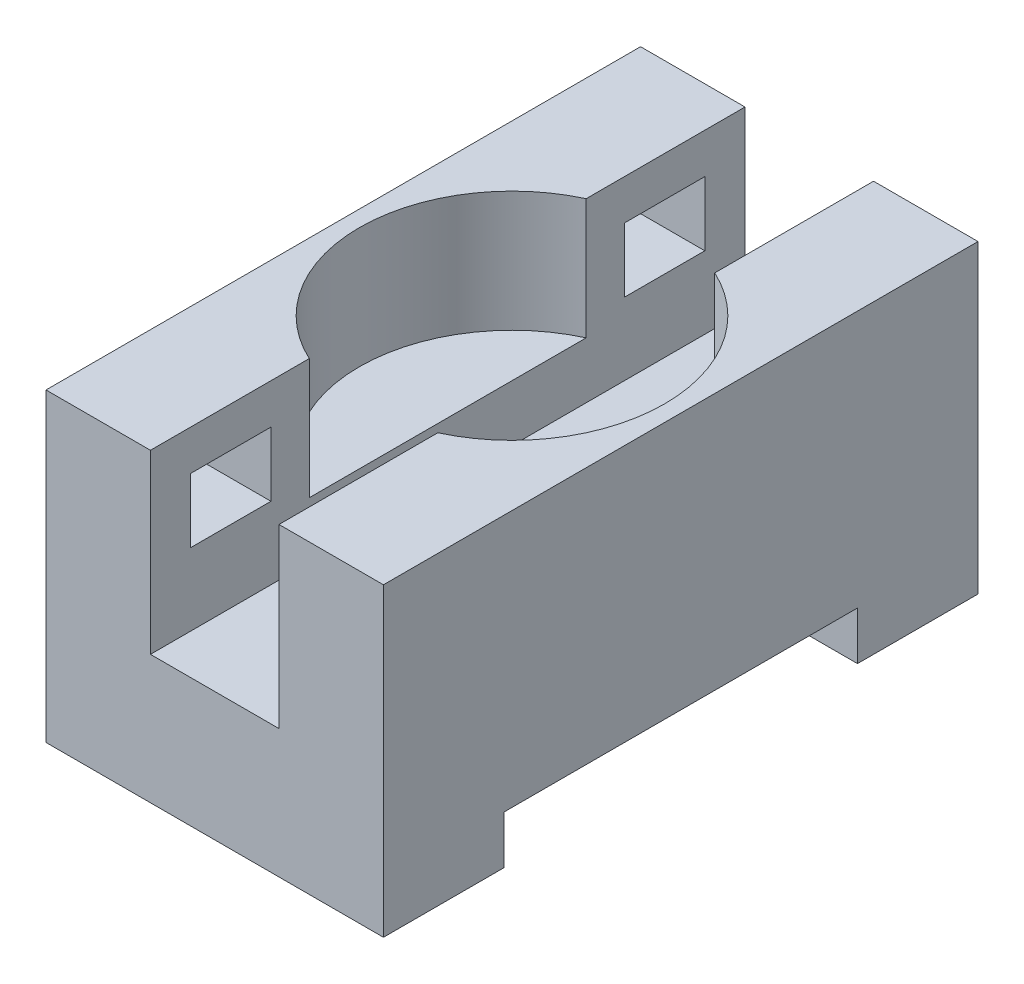
ISO-10303-21;
HEADER;
FILE_DESCRIPTION(('STEP AP214'),'2;1');
FILE_NAME('part.step','',(''),(''),'','','');
FILE_SCHEMA(('AUTOMOTIVE_DESIGN { 1 0 10303 214 1 1 1 1 }'));
ENDSEC;
DATA;
#1=APPLICATION_CONTEXT('core data for automotive mechanical design processes');
#2=APPLICATION_PROTOCOL_DEFINITION('international standard','automotive_design',2000,#1);
#3=PRODUCT_CONTEXT('',#1,'mechanical');
#4=PRODUCT('Part','Part','',(#3));
#5=PRODUCT_RELATED_PRODUCT_CATEGORY('part','',(#4));
#6=PRODUCT_DEFINITION_FORMATION('','',#4);
#7=PRODUCT_DEFINITION_CONTEXT('part definition',#1,'design');
#8=PRODUCT_DEFINITION('design','',#6,#7);
#9=PRODUCT_DEFINITION_SHAPE('','',#8);
#10=(LENGTH_UNIT() NAMED_UNIT(*) SI_UNIT(.MILLI.,.METRE.));
#11=(NAMED_UNIT(*) PLANE_ANGLE_UNIT() SI_UNIT($,.RADIAN.));
#12=(NAMED_UNIT(*) SI_UNIT($,.STERADIAN.) SOLID_ANGLE_UNIT());
#13=UNCERTAINTY_MEASURE_WITH_UNIT(LENGTH_MEASURE(1.E-05),#10,'distance_accuracy_value','');
#14=(GEOMETRIC_REPRESENTATION_CONTEXT(3) GLOBAL_UNCERTAINTY_ASSIGNED_CONTEXT((#13)) GLOBAL_UNIT_ASSIGNED_CONTEXT((#10,
#11,#12)) REPRESENTATION_CONTEXT('',''));
#15=CARTESIAN_POINT('',(0.,0.,0.));
#16=DIRECTION('',(0.,0.,1.));
#17=DIRECTION('',(1.,0.,0.));
#18=AXIS2_PLACEMENT_3D('',#15,#16,#17);
#19=CARTESIAN_POINT('',(-21.,0.,-74.));
#20=DIRECTION('',(0.,-1.,0.));
#21=DIRECTION('',(0.,0.,-1.));
#22=AXIS2_PLACEMENT_3D('',#19,#20,#21);
#23=PLANE('',#22);
#24=DIRECTION('',(1.,0.,0.));
#25=VECTOR('',#24,1.);
#26=CARTESIAN_POINT('',(-21.,0.,-15.));
#27=LINE('',#26,#25);
#28=CARTESIAN_POINT('',(-21.,0.,-15.));
#29=VERTEX_POINT('',#28);
#30=CARTESIAN_POINT('',(21.,0.,-15.));
#31=VERTEX_POINT('',#30);
#32=EDGE_CURVE('E420',#29,#31,#27,.T.);
#33=ORIENTED_EDGE('',*,*,#32,.T.);
#34=DIRECTION('',(0.,0.,1.));
#35=VECTOR('',#34,1.);
#36=CARTESIAN_POINT('',(21.,0.,-74.));
#37=LINE('',#36,#35);
#38=CARTESIAN_POINT('',(21.,0.,0.));
#39=VERTEX_POINT('',#38);
#40=EDGE_CURVE('E476',#31,#39,#37,.T.);
#41=ORIENTED_EDGE('',*,*,#40,.T.);
#42=DIRECTION('',(1.,0.,0.));
#43=VECTOR('',#42,1.);
#44=CARTESIAN_POINT('',(-21.,0.,0.));
#45=LINE('',#44,#43);
#46=CARTESIAN_POINT('',(-21.,0.,0.));
#47=VERTEX_POINT('',#46);
#48=EDGE_CURVE('E435',#47,#39,#45,.T.);
#49=ORIENTED_EDGE('',*,*,#48,.F.);
#50=DIRECTION('',(0.,0.,1.));
#51=VECTOR('',#50,1.);
#52=CARTESIAN_POINT('',(-21.,0.,-74.));
#53=LINE('',#52,#51);
#54=EDGE_CURVE('E485',#29,#47,#53,.T.);
#55=ORIENTED_EDGE('',*,*,#54,.F.);
#56=EDGE_LOOP('',(#33,#41,#49,#55));
#57=FACE_BOUND('',#56,.T.);
#58=ADVANCED_FACE('F41',(#57),#23,.T.);
#59=CARTESIAN_POINT('',(21.,0.,-74.));
#60=DIRECTION('',(1.,0.,0.));
#61=DIRECTION('',(0.,0.,-1.));
#62=AXIS2_PLACEMENT_3D('',#59,#60,#61);
#63=PLANE('',#62);
#64=DIRECTION('',(0.,-1.,0.));
#65=VECTOR('',#64,1.);
#66=CARTESIAN_POINT('',(21.,0.,-15.));
#67=LINE('',#66,#65);
#68=CARTESIAN_POINT('',(21.,6.,-15.));
#69=VERTEX_POINT('',#68);
#70=EDGE_CURVE('E407',#69,#31,#67,.T.);
#71=ORIENTED_EDGE('',*,*,#70,.F.);
#72=DIRECTION('',(0.,0.,1.));
#73=VECTOR('',#72,1.);
#74=CARTESIAN_POINT('',(21.,6.,-15.));
#75=LINE('',#74,#73);
#76=CARTESIAN_POINT('',(21.,6.,-59.));
#77=VERTEX_POINT('',#76);
#78=EDGE_CURVE('E413',#77,#69,#75,.T.);
#79=ORIENTED_EDGE('',*,*,#78,.F.);
#80=DIRECTION('',(0.,1.,0.));
#81=VECTOR('',#80,1.);
#82=CARTESIAN_POINT('',(21.,6.,-59.));
#83=LINE('',#82,#81);
#84=CARTESIAN_POINT('',(21.,0.,-59.));
#85=VERTEX_POINT('',#84);
#86=EDGE_CURVE('E402',#85,#77,#83,.T.);
#87=ORIENTED_EDGE('',*,*,#86,.F.);
#88=CARTESIAN_POINT('',(21.,0.,-74.));
#89=VERTEX_POINT('',#88);
#90=EDGE_CURVE('E47',#89,#85,#37,.T.);
#91=ORIENTED_EDGE('',*,*,#90,.F.);
#92=DIRECTION('',(0.,1.,0.));
#93=VECTOR('',#92,1.);
#94=CARTESIAN_POINT('',(21.,0.,-74.));
#95=LINE('',#94,#93);
#96=CARTESIAN_POINT('',(21.,38.,-74.));
#97=VERTEX_POINT('',#96);
#98=EDGE_CURVE('E428',#89,#97,#95,.T.);
#99=ORIENTED_EDGE('',*,*,#98,.T.);
#100=DIRECTION('',(0.,0.,1.));
#101=VECTOR('',#100,1.);
#102=CARTESIAN_POINT('',(21.,38.,-74.));
#103=LINE('',#102,#101);
#104=CARTESIAN_POINT('',(21.,38.,0.));
#105=VERTEX_POINT('',#104);
#106=EDGE_CURVE('E454',#97,#105,#103,.T.);
#107=ORIENTED_EDGE('',*,*,#106,.T.);
#108=DIRECTION('',(0.,1.,0.));
#109=VECTOR('',#108,1.);
#110=CARTESIAN_POINT('',(21.,0.,0.));
#111=LINE('',#110,#109);
#112=EDGE_CURVE('E425',#39,#105,#111,.T.);
#113=ORIENTED_EDGE('',*,*,#112,.F.);
#114=ORIENTED_EDGE('',*,*,#40,.F.);
#115=EDGE_LOOP('',(#71,#79,#87,#91,#99,#107,#113,#114));
#116=FACE_BOUND('',#115,.T.);
#117=ADVANCED_FACE('F43',(#116),#63,.T.);
#118=DIRECTION('',(1.,0.,0.));
#119=VECTOR('',#118,1.);
#120=CARTESIAN_POINT('',(-21.,0.,-59.));
#121=LINE('',#120,#119);
#122=CARTESIAN_POINT('',(-21.,0.,-59.));
#123=VERTEX_POINT('',#122);
#124=EDGE_CURVE('E415',#123,#85,#121,.T.);
#125=ORIENTED_EDGE('',*,*,#124,.F.);
#126=CARTESIAN_POINT('',(-21.,0.,-74.));
#127=VERTEX_POINT('',#126);
#128=EDGE_CURVE('E479',#127,#123,#53,.T.);
#129=ORIENTED_EDGE('',*,*,#128,.F.);
#130=DIRECTION('',(1.,0.,0.));
#131=VECTOR('',#130,1.);
#132=CARTESIAN_POINT('',(-21.,0.,-74.));
#133=LINE('',#132,#131);
#134=EDGE_CURVE('E448',#127,#89,#133,.T.);
#135=ORIENTED_EDGE('',*,*,#134,.T.);
#136=ORIENTED_EDGE('',*,*,#90,.T.);
#137=EDGE_LOOP('',(#125,#129,#135,#136));
#138=FACE_BOUND('',#137,.T.);
#139=ADVANCED_FACE('F533',(#138),#23,.T.);
#140=CARTESIAN_POINT('',(-21.,38.,-74.));
#141=DIRECTION('',(-1.,0.,0.));
#142=DIRECTION('',(0.,-1.,0.));
#143=AXIS2_PLACEMENT_3D('',#140,#141,#142);
#144=PLANE('',#143);
#145=DIRECTION('',(0.,-1.,0.));
#146=VECTOR('',#145,1.);
#147=CARTESIAN_POINT('',(-21.,0.,-15.));
#148=LINE('',#147,#146);
#149=CARTESIAN_POINT('',(-21.,6.,-15.));
#150=VERTEX_POINT('',#149);
#151=EDGE_CURVE('E406',#150,#29,#148,.T.);
#152=ORIENTED_EDGE('',*,*,#151,.T.);
#153=ORIENTED_EDGE('',*,*,#54,.T.);
#154=DIRECTION('',(0.,-1.,0.));
#155=VECTOR('',#154,1.);
#156=CARTESIAN_POINT('',(-21.,38.,0.));
#157=LINE('',#156,#155);
#158=CARTESIAN_POINT('',(-21.,38.,0.));
#159=VERTEX_POINT('',#158);
#160=EDGE_CURVE('E473',#159,#47,#157,.T.);
#161=ORIENTED_EDGE('',*,*,#160,.F.);
#162=DIRECTION('',(0.,0.,1.));
#163=VECTOR('',#162,1.);
#164=CARTESIAN_POINT('',(-21.,38.,-74.));
#165=LINE('',#164,#163);
#166=CARTESIAN_POINT('',(-21.,38.,-74.));
#167=VERTEX_POINT('',#166);
#168=EDGE_CURVE('E483',#167,#159,#165,.T.);
#169=ORIENTED_EDGE('',*,*,#168,.F.);
#170=DIRECTION('',(0.,-1.,0.));
#171=VECTOR('',#170,1.);
#172=CARTESIAN_POINT('',(-21.,38.,-74.));
#173=LINE('',#172,#171);
#174=EDGE_CURVE('E449',#167,#127,#173,.T.);
#175=ORIENTED_EDGE('',*,*,#174,.T.);
#176=ORIENTED_EDGE('',*,*,#128,.T.);
#177=DIRECTION('',(0.,1.,0.));
#178=VECTOR('',#177,1.);
#179=CARTESIAN_POINT('',(-21.,6.,-59.));
#180=LINE('',#179,#178);
#181=CARTESIAN_POINT('',(-21.,6.,-59.));
#182=VERTEX_POINT('',#181);
#183=EDGE_CURVE('E405',#123,#182,#180,.T.);
#184=ORIENTED_EDGE('',*,*,#183,.T.);
#185=DIRECTION('',(0.,0.,1.));
#186=VECTOR('',#185,1.);
#187=CARTESIAN_POINT('',(-21.,6.,-15.));
#188=LINE('',#187,#186);
#189=EDGE_CURVE('E403',#182,#150,#188,.T.);
#190=ORIENTED_EDGE('',*,*,#189,.T.);
#191=EDGE_LOOP('',(#152,#153,#161,#169,#175,#176,#184,#190));
#192=FACE_BOUND('',#191,.T.);
#193=ADVANCED_FACE('F518',(#192),#144,.T.);
#194=CARTESIAN_POINT('',(-7.99999999999999,38.,-74.));
#195=DIRECTION('',(0.,1.,0.));
#196=DIRECTION('',(0.,0.,1.));
#197=AXIS2_PLACEMENT_3D('',#194,#195,#196);
#198=PLANE('',#197);
#199=CARTESIAN_POINT('',(0.,38.,-37.));
#200=DIRECTION('',(0.,1.,0.));
#201=DIRECTION('',(0.,0.,1.));
#202=AXIS2_PLACEMENT_3D('',#199,#200,#201);
#203=CIRCLE('',#202,19.);
#204=CARTESIAN_POINT('',(-7.99999999999999,38.,-54.2336879396141));
#205=VERTEX_POINT('',#204);
#206=CARTESIAN_POINT('',(-7.99999999999999,38.,-19.7663120603859));
#207=VERTEX_POINT('',#206);
#208=EDGE_CURVE('E347',#205,#207,#203,.T.);
#209=ORIENTED_EDGE('',*,*,#208,.F.);
#210=DIRECTION('',(0.,0.,1.));
#211=VECTOR('',#210,1.);
#212=CARTESIAN_POINT('',(-7.99999999999999,38.,-74.));
#213=LINE('',#212,#211);
#214=CARTESIAN_POINT('',(-7.99999999999999,38.,-74.));
#215=VERTEX_POINT('',#214);
#216=EDGE_CURVE('E484',#215,#205,#213,.T.);
#217=ORIENTED_EDGE('',*,*,#216,.F.);
#218=DIRECTION('',(-1.,0.,0.));
#219=VECTOR('',#218,1.);
#220=CARTESIAN_POINT('',(-7.99999999999999,38.,-74.));
#221=LINE('',#220,#219);
#222=EDGE_CURVE('E441',#215,#167,#221,.T.);
#223=ORIENTED_EDGE('',*,*,#222,.T.);
#224=ORIENTED_EDGE('',*,*,#168,.T.);
#225=DIRECTION('',(-1.,0.,0.));
#226=VECTOR('',#225,1.);
#227=CARTESIAN_POINT('',(-7.99999999999999,38.,0.));
#228=LINE('',#227,#226);
#229=CARTESIAN_POINT('',(-7.99999999999999,38.,0.));
#230=VERTEX_POINT('',#229);
#231=EDGE_CURVE('E469',#230,#159,#228,.T.);
#232=ORIENTED_EDGE('',*,*,#231,.F.);
#233=EDGE_CURVE('E488',#207,#230,#213,.T.);
#234=ORIENTED_EDGE('',*,*,#233,.F.);
#235=EDGE_LOOP('',(#209,#217,#223,#224,#232,#234));
#236=FACE_BOUND('',#235,.T.);
#237=ADVANCED_FACE('F569',(#236),#198,.T.);
#238=CARTESIAN_POINT('',(-7.99999999999999,16.,-74.));
#239=DIRECTION('',(1.,0.,0.));
#240=DIRECTION('',(0.,0.,-1.));
#241=AXIS2_PLACEMENT_3D('',#238,#239,#240);
#242=PLANE('',#241);
#243=DIRECTION('',(0.,-1.,0.));
#244=VECTOR('',#243,1.);
#245=CARTESIAN_POINT('',(-7.99999999999999,25.,-5.));
#246=LINE('',#245,#244);
#247=CARTESIAN_POINT('',(-7.99999999999999,33.,-5.));
#248=VERTEX_POINT('',#247);
#249=CARTESIAN_POINT('',(-7.99999999999999,25.,-5.));
#250=VERTEX_POINT('',#249);
#251=EDGE_CURVE('E334',#248,#250,#246,.T.);
#252=ORIENTED_EDGE('',*,*,#251,.F.);
#253=DIRECTION('',(0.,0.,1.));
#254=VECTOR('',#253,1.);
#255=CARTESIAN_POINT('',(-7.99999999999999,33.,-5.));
#256=LINE('',#255,#254);
#257=CARTESIAN_POINT('',(-7.99999999999999,33.,-15.));
#258=VERTEX_POINT('',#257);
#259=EDGE_CURVE('E323',#258,#248,#256,.T.);
#260=ORIENTED_EDGE('',*,*,#259,.F.);
#261=DIRECTION('',(0.,1.,0.));
#262=VECTOR('',#261,1.);
#263=CARTESIAN_POINT('',(-7.99999999999999,25.,-15.));
#264=LINE('',#263,#262);
#265=CARTESIAN_POINT('',(-7.99999999999999,25.,-15.));
#266=VERTEX_POINT('',#265);
#267=EDGE_CURVE('E336',#266,#258,#264,.T.);
#268=ORIENTED_EDGE('',*,*,#267,.F.);
#269=DIRECTION('',(0.,0.,-1.));
#270=VECTOR('',#269,1.);
#271=CARTESIAN_POINT('',(-7.99999999999999,25.,-5.));
#272=LINE('',#271,#270);
#273=EDGE_CURVE('E333',#250,#266,#272,.T.);
#274=ORIENTED_EDGE('',*,*,#273,.F.);
#275=EDGE_LOOP('',(#252,#260,#268,#274));
#276=FACE_BOUND('',#275,.T.);
#277=DIRECTION('',(0.,0.,-1.));
#278=VECTOR('',#277,1.);
#279=CARTESIAN_POINT('',(-7.99999999999999,25.,-69.));
#280=LINE('',#279,#278);
#281=CARTESIAN_POINT('',(-7.99999999999999,25.,-59.));
#282=VERTEX_POINT('',#281);
#283=CARTESIAN_POINT('',(-7.99999999999999,25.,-69.));
#284=VERTEX_POINT('',#283);
#285=EDGE_CURVE('E337',#282,#284,#280,.T.);
#286=ORIENTED_EDGE('',*,*,#285,.F.);
#287=DIRECTION('',(0.,-1.,0.));
#288=VECTOR('',#287,1.);
#289=CARTESIAN_POINT('',(-7.99999999999999,25.,-59.));
#290=LINE('',#289,#288);
#291=CARTESIAN_POINT('',(-7.99999999999999,33.,-59.));
#292=VERTEX_POINT('',#291);
#293=EDGE_CURVE('E362',#292,#282,#290,.T.);
#294=ORIENTED_EDGE('',*,*,#293,.F.);
#295=DIRECTION('',(0.,0.,1.));
#296=VECTOR('',#295,1.);
#297=CARTESIAN_POINT('',(-7.99999999999999,33.,-69.));
#298=LINE('',#297,#296);
#299=CARTESIAN_POINT('',(-7.99999999999999,33.,-69.));
#300=VERTEX_POINT('',#299);
#301=EDGE_CURVE('E364',#300,#292,#298,.T.);
#302=ORIENTED_EDGE('',*,*,#301,.F.);
#303=DIRECTION('',(0.,1.,0.));
#304=VECTOR('',#303,1.);
#305=CARTESIAN_POINT('',(-7.99999999999999,25.,-69.));
#306=LINE('',#305,#304);
#307=EDGE_CURVE('E369',#284,#300,#306,.T.);
#308=ORIENTED_EDGE('',*,*,#307,.F.);
#309=EDGE_LOOP('',(#286,#294,#302,#308));
#310=FACE_BOUND('',#309,.T.);
#311=DIRECTION('',(0.,1.,0.));
#312=VECTOR('',#311,1.);
#313=CARTESIAN_POINT('',(-7.99999999999999,23.,-54.2336879396141));
#314=LINE('',#313,#312);
#315=CARTESIAN_POINT('',(-7.99999999999999,23.,-54.2336879396141));
#316=VERTEX_POINT('',#315);
#317=EDGE_CURVE('E397',#316,#205,#314,.T.);
#318=ORIENTED_EDGE('',*,*,#317,.F.);
#319=DIRECTION('',(0.,0.,1.));
#320=VECTOR('',#319,1.);
#321=CARTESIAN_POINT('',(-7.99999999999999,23.,-74.));
#322=LINE('',#321,#320);
#323=CARTESIAN_POINT('',(-7.99999999999999,23.,-19.7663120603859));
#324=VERTEX_POINT('',#323);
#325=EDGE_CURVE('E399',#316,#324,#322,.T.);
#326=ORIENTED_EDGE('',*,*,#325,.T.);
#327=DIRECTION('',(0.,1.,0.));
#328=VECTOR('',#327,1.);
#329=CARTESIAN_POINT('',(-7.99999999999999,23.,-19.7663120603859));
#330=LINE('',#329,#328);
#331=EDGE_CURVE('E395',#207,#324,#330,.F.);
#332=ORIENTED_EDGE('',*,*,#331,.F.);
#333=ORIENTED_EDGE('',*,*,#233,.T.);
#334=DIRECTION('',(0.,1.,0.));
#335=VECTOR('',#334,1.);
#336=CARTESIAN_POINT('',(-7.99999999999999,16.,0.));
#337=LINE('',#336,#335);
#338=CARTESIAN_POINT('',(-7.99999999999999,16.,0.));
#339=VERTEX_POINT('',#338);
#340=EDGE_CURVE('E463',#339,#230,#337,.T.);
#341=ORIENTED_EDGE('',*,*,#340,.F.);
#342=DIRECTION('',(0.,0.,1.));
#343=VECTOR('',#342,1.);
#344=CARTESIAN_POINT('',(-7.99999999999999,16.,-74.));
#345=LINE('',#344,#343);
#346=CARTESIAN_POINT('',(-7.99999999999999,16.,-74.));
#347=VERTEX_POINT('',#346);
#348=EDGE_CURVE('E487',#347,#339,#345,.T.);
#349=ORIENTED_EDGE('',*,*,#348,.F.);
#350=DIRECTION('',(0.,1.,0.));
#351=VECTOR('',#350,1.);
#352=CARTESIAN_POINT('',(-7.99999999999999,16.,-74.));
#353=LINE('',#352,#351);
#354=EDGE_CURVE('E442',#347,#215,#353,.T.);
#355=ORIENTED_EDGE('',*,*,#354,.T.);
#356=ORIENTED_EDGE('',*,*,#216,.T.);
#357=EDGE_LOOP('',(#318,#326,#332,#333,#341,#349,#355,#356));
#358=FACE_BOUND('',#357,.T.);
#359=ADVANCED_FACE('F571',(#276,#310,#358),#242,.T.);
#360=CARTESIAN_POINT('',(8.00000000000001,16.,-74.));
#361=DIRECTION('',(0.,1.,0.));
#362=DIRECTION('',(-1.,0.,0.));
#363=AXIS2_PLACEMENT_3D('',#360,#361,#362);
#364=PLANE('',#363);
#365=DIRECTION('',(-1.,0.,0.));
#366=VECTOR('',#365,1.);
#367=CARTESIAN_POINT('',(8.00000000000001,16.,0.));
#368=LINE('',#367,#366);
#369=CARTESIAN_POINT('',(8.00000000000001,16.,0.));
#370=VERTEX_POINT('',#369);
#371=EDGE_CURVE('E464',#370,#339,#368,.T.);
#372=ORIENTED_EDGE('',*,*,#371,.F.);
#373=DIRECTION('',(0.,0.,1.));
#374=VECTOR('',#373,1.);
#375=CARTESIAN_POINT('',(8.00000000000001,16.,-74.));
#376=LINE('',#375,#374);
#377=CARTESIAN_POINT('',(8.00000000000001,16.,-74.));
#378=VERTEX_POINT('',#377);
#379=EDGE_CURVE('E491',#378,#370,#376,.T.);
#380=ORIENTED_EDGE('',*,*,#379,.F.);
#381=DIRECTION('',(-1.,0.,0.));
#382=VECTOR('',#381,1.);
#383=CARTESIAN_POINT('',(8.00000000000001,16.,-74.));
#384=LINE('',#383,#382);
#385=EDGE_CURVE('E437',#378,#347,#384,.T.);
#386=ORIENTED_EDGE('',*,*,#385,.T.);
#387=ORIENTED_EDGE('',*,*,#348,.T.);
#388=EDGE_LOOP('',(#372,#380,#386,#387));
#389=FACE_BOUND('',#388,.T.);
#390=ADVANCED_FACE('F578',(#389),#364,.T.);
#391=CARTESIAN_POINT('',(8.,38.,-74.));
#392=DIRECTION('',(-1.,0.,0.));
#393=DIRECTION('',(0.,-1.,0.));
#394=AXIS2_PLACEMENT_3D('',#391,#392,#393);
#395=PLANE('',#394);
#396=DIRECTION('',(0.,-1.,0.));
#397=VECTOR('',#396,1.);
#398=CARTESIAN_POINT('',(8.,25.,-69.));
#399=LINE('',#398,#397);
#400=CARTESIAN_POINT('',(8.,33.,-69.));
#401=VERTEX_POINT('',#400);
#402=CARTESIAN_POINT('',(8.,25.,-69.));
#403=VERTEX_POINT('',#402);
#404=EDGE_CURVE('E57',#401,#403,#399,.T.);
#405=ORIENTED_EDGE('',*,*,#404,.F.);
#406=DIRECTION('',(0.,0.,-1.));
#407=VECTOR('',#406,1.);
#408=CARTESIAN_POINT('',(8.,33.,-69.));
#409=LINE('',#408,#407);
#410=CARTESIAN_POINT('',(8.,33.,-59.));
#411=VERTEX_POINT('',#410);
#412=EDGE_CURVE('E269',#411,#401,#409,.T.);
#413=ORIENTED_EDGE('',*,*,#412,.F.);
#414=DIRECTION('',(0.,1.,0.));
#415=VECTOR('',#414,1.);
#416=CARTESIAN_POINT('',(8.,25.,-59.));
#417=LINE('',#416,#415);
#418=CARTESIAN_POINT('',(8.,25.,-59.));
#419=VERTEX_POINT('',#418);
#420=EDGE_CURVE('E272',#419,#411,#417,.T.);
#421=ORIENTED_EDGE('',*,*,#420,.F.);
#422=DIRECTION('',(0.,0.,1.));
#423=VECTOR('',#422,1.);
#424=CARTESIAN_POINT('',(8.,25.,-69.));
#425=LINE('',#424,#423);
#426=EDGE_CURVE('E276',#403,#419,#425,.T.);
#427=ORIENTED_EDGE('',*,*,#426,.F.);
#428=EDGE_LOOP('',(#405,#413,#421,#427));
#429=FACE_BOUND('',#428,.T.);
#430=DIRECTION('',(0.,0.,1.));
#431=VECTOR('',#430,1.);
#432=CARTESIAN_POINT('',(8.,25.,-5.));
#433=LINE('',#432,#431);
#434=CARTESIAN_POINT('',(8.,25.,-15.));
#435=VERTEX_POINT('',#434);
#436=CARTESIAN_POINT('',(8.,25.,-5.));
#437=VERTEX_POINT('',#436);
#438=EDGE_CURVE('E61',#435,#437,#433,.T.);
#439=ORIENTED_EDGE('',*,*,#438,.F.);
#440=DIRECTION('',(0.,-1.,0.));
#441=VECTOR('',#440,1.);
#442=CARTESIAN_POINT('',(8.,25.,-15.));
#443=LINE('',#442,#441);
#444=CARTESIAN_POINT('',(8.,33.,-15.));
#445=VERTEX_POINT('',#444);
#446=EDGE_CURVE('E300',#445,#435,#443,.T.);
#447=ORIENTED_EDGE('',*,*,#446,.F.);
#448=DIRECTION('',(0.,0.,-1.));
#449=VECTOR('',#448,1.);
#450=CARTESIAN_POINT('',(8.,33.,-5.));
#451=LINE('',#450,#449);
#452=CARTESIAN_POINT('',(8.,33.,-5.));
#453=VERTEX_POINT('',#452);
#454=EDGE_CURVE('E302',#453,#445,#451,.T.);
#455=ORIENTED_EDGE('',*,*,#454,.F.);
#456=DIRECTION('',(0.,1.,0.));
#457=VECTOR('',#456,1.);
#458=CARTESIAN_POINT('',(8.,25.,-5.));
#459=LINE('',#458,#457);
#460=EDGE_CURVE('E303',#437,#453,#459,.T.);
#461=ORIENTED_EDGE('',*,*,#460,.F.);
#462=EDGE_LOOP('',(#439,#447,#455,#461));
#463=FACE_BOUND('',#462,.T.);
#464=DIRECTION('',(0.,1.,0.));
#465=VECTOR('',#464,1.);
#466=CARTESIAN_POINT('',(8.,23.,-19.7663120603859));
#467=LINE('',#466,#465);
#468=CARTESIAN_POINT('',(8.,23.,-19.7663120603859));
#469=VERTEX_POINT('',#468);
#470=CARTESIAN_POINT('',(8.,38.,-19.7663120603859));
#471=VERTEX_POINT('',#470);
#472=EDGE_CURVE('E392',#469,#471,#467,.T.);
#473=ORIENTED_EDGE('',*,*,#472,.F.);
#474=DIRECTION('',(0.,0.,-1.));
#475=VECTOR('',#474,1.);
#476=CARTESIAN_POINT('',(8.,23.,-74.));
#477=LINE('',#476,#475);
#478=CARTESIAN_POINT('',(8.,23.,-54.2336879396141));
#479=VERTEX_POINT('',#478);
#480=EDGE_CURVE('E11',#469,#479,#477,.T.);
#481=ORIENTED_EDGE('',*,*,#480,.T.);
#482=DIRECTION('',(0.,1.,0.));
#483=VECTOR('',#482,1.);
#484=CARTESIAN_POINT('',(8.,23.,-54.2336879396141));
#485=LINE('',#484,#483);
#486=CARTESIAN_POINT('',(8.,38.,-54.2336879396141));
#487=VERTEX_POINT('',#486);
#488=EDGE_CURVE('E387',#487,#479,#485,.F.);
#489=ORIENTED_EDGE('',*,*,#488,.F.);
#490=DIRECTION('',(0.,0.,1.));
#491=VECTOR('',#490,1.);
#492=CARTESIAN_POINT('',(8.,38.,-74.));
#493=LINE('',#492,#491);
#494=CARTESIAN_POINT('',(8.,38.,-74.));
#495=VERTEX_POINT('',#494);
#496=EDGE_CURVE('E492',#495,#487,#493,.T.);
#497=ORIENTED_EDGE('',*,*,#496,.F.);
#498=DIRECTION('',(0.,-1.,0.));
#499=VECTOR('',#498,1.);
#500=CARTESIAN_POINT('',(8.,38.,-74.));
#501=LINE('',#500,#499);
#502=EDGE_CURVE('E434',#495,#378,#501,.T.);
#503=ORIENTED_EDGE('',*,*,#502,.T.);
#504=ORIENTED_EDGE('',*,*,#379,.T.);
#505=DIRECTION('',(0.,-1.,0.));
#506=VECTOR('',#505,1.);
#507=CARTESIAN_POINT('',(8.,38.,0.));
#508=LINE('',#507,#506);
#509=CARTESIAN_POINT('',(8.,38.,0.));
#510=VERTEX_POINT('',#509);
#511=EDGE_CURVE('E459',#510,#370,#508,.T.);
#512=ORIENTED_EDGE('',*,*,#511,.F.);
#513=EDGE_CURVE('E494',#471,#510,#493,.T.);
#514=ORIENTED_EDGE('',*,*,#513,.F.);
#515=EDGE_LOOP('',(#473,#481,#489,#497,#503,#504,#512,#514));
#516=FACE_BOUND('',#515,.T.);
#517=ADVANCED_FACE('F507',(#429,#463,#516),#395,.T.);
#518=CARTESIAN_POINT('',(21.,38.,-74.));
#519=DIRECTION('',(0.,1.,0.));
#520=DIRECTION('',(0.,0.,1.));
#521=AXIS2_PLACEMENT_3D('',#518,#519,#520);
#522=PLANE('',#521);
#523=EDGE_CURVE('E389',#471,#487,#203,.T.);
#524=ORIENTED_EDGE('',*,*,#523,.F.);
#525=ORIENTED_EDGE('',*,*,#513,.T.);
#526=DIRECTION('',(-1.,0.,0.));
#527=VECTOR('',#526,1.);
#528=CARTESIAN_POINT('',(21.,38.,0.));
#529=LINE('',#528,#527);
#530=EDGE_CURVE('E457',#105,#510,#529,.T.);
#531=ORIENTED_EDGE('',*,*,#530,.F.);
#532=ORIENTED_EDGE('',*,*,#106,.F.);
#533=DIRECTION('',(-1.,0.,0.));
#534=VECTOR('',#533,1.);
#535=CARTESIAN_POINT('',(21.,38.,-74.));
#536=LINE('',#535,#534);
#537=EDGE_CURVE('E431',#97,#495,#536,.T.);
#538=ORIENTED_EDGE('',*,*,#537,.T.);
#539=ORIENTED_EDGE('',*,*,#496,.T.);
#540=EDGE_LOOP('',(#524,#525,#531,#532,#538,#539));
#541=FACE_BOUND('',#540,.T.);
#542=ADVANCED_FACE('F505',(#541),#522,.T.);
#543=CARTESIAN_POINT('',(0.,0.,-74.));
#544=DIRECTION('',(0.,0.,1.));
#545=DIRECTION('',(1.,0.,0.));
#546=AXIS2_PLACEMENT_3D('',#543,#544,#545);
#547=PLANE('',#546);
#548=ORIENTED_EDGE('',*,*,#98,.F.);
#549=ORIENTED_EDGE('',*,*,#134,.F.);
#550=ORIENTED_EDGE('',*,*,#174,.F.);
#551=ORIENTED_EDGE('',*,*,#222,.F.);
#552=ORIENTED_EDGE('',*,*,#354,.F.);
#553=ORIENTED_EDGE('',*,*,#385,.F.);
#554=ORIENTED_EDGE('',*,*,#502,.F.);
#555=ORIENTED_EDGE('',*,*,#537,.F.);
#556=EDGE_LOOP('',(#548,#549,#550,#551,#552,#553,#554,#555));
#557=FACE_BOUND('',#556,.T.);
#558=ADVANCED_FACE('F532',(#557),#547,.F.);
#559=CARTESIAN_POINT('',(0.,0.,0.));
#560=DIRECTION('',(0.,0.,1.));
#561=DIRECTION('',(1.,0.,0.));
#562=AXIS2_PLACEMENT_3D('',#559,#560,#561);
#563=PLANE('',#562);
#564=ORIENTED_EDGE('',*,*,#112,.T.);
#565=ORIENTED_EDGE('',*,*,#530,.T.);
#566=ORIENTED_EDGE('',*,*,#511,.T.);
#567=ORIENTED_EDGE('',*,*,#371,.T.);
#568=ORIENTED_EDGE('',*,*,#340,.T.);
#569=ORIENTED_EDGE('',*,*,#231,.T.);
#570=ORIENTED_EDGE('',*,*,#160,.T.);
#571=ORIENTED_EDGE('',*,*,#48,.T.);
#572=EDGE_LOOP('',(#564,#565,#566,#567,#568,#569,#570,#571));
#573=FACE_BOUND('',#572,.T.);
#574=ADVANCED_FACE('F506',(#573),#563,.T.);
#575=CARTESIAN_POINT('',(-21.,0.,-15.));
#576=DIRECTION('',(0.,0.,1.));
#577=DIRECTION('',(1.,0.,0.));
#578=AXIS2_PLACEMENT_3D('',#575,#576,#577);
#579=PLANE('',#578);
#580=ORIENTED_EDGE('',*,*,#70,.T.);
#581=ORIENTED_EDGE('',*,*,#32,.F.);
#582=ORIENTED_EDGE('',*,*,#151,.F.);
#583=DIRECTION('',(1.,0.,0.));
#584=VECTOR('',#583,1.);
#585=CARTESIAN_POINT('',(-21.,6.,-15.));
#586=LINE('',#585,#584);
#587=EDGE_CURVE('E421',#150,#69,#586,.T.);
#588=ORIENTED_EDGE('',*,*,#587,.T.);
#589=EDGE_LOOP('',(#580,#581,#582,#588));
#590=FACE_BOUND('',#589,.T.);
#591=ADVANCED_FACE('F520',(#590),#579,.F.);
#592=CARTESIAN_POINT('',(-21.,6.,-15.));
#593=DIRECTION('',(0.,1.,0.));
#594=DIRECTION('',(0.,0.,1.));
#595=AXIS2_PLACEMENT_3D('',#592,#593,#594);
#596=PLANE('',#595);
#597=ORIENTED_EDGE('',*,*,#78,.T.);
#598=ORIENTED_EDGE('',*,*,#587,.F.);
#599=ORIENTED_EDGE('',*,*,#189,.F.);
#600=DIRECTION('',(1.,0.,0.));
#601=VECTOR('',#600,1.);
#602=CARTESIAN_POINT('',(-21.,6.,-59.));
#603=LINE('',#602,#601);
#604=EDGE_CURVE('E422',#182,#77,#603,.T.);
#605=ORIENTED_EDGE('',*,*,#604,.T.);
#606=EDGE_LOOP('',(#597,#598,#599,#605));
#607=FACE_BOUND('',#606,.T.);
#608=ADVANCED_FACE('F521',(#607),#596,.F.);
#609=CARTESIAN_POINT('',(-21.,6.,-59.));
#610=DIRECTION('',(0.,0.,-1.));
#611=DIRECTION('',(-1.,0.,0.));
#612=AXIS2_PLACEMENT_3D('',#609,#610,#611);
#613=PLANE('',#612);
#614=ORIENTED_EDGE('',*,*,#86,.T.);
#615=ORIENTED_EDGE('',*,*,#604,.F.);
#616=ORIENTED_EDGE('',*,*,#183,.F.);
#617=ORIENTED_EDGE('',*,*,#124,.T.);
#618=EDGE_LOOP('',(#614,#615,#616,#617));
#619=FACE_BOUND('',#618,.T.);
#620=ADVANCED_FACE('F528',(#619),#613,.F.);
#621=CARTESIAN_POINT('',(0.,23.,-37.));
#622=DIRECTION('',(0.,1.,0.));
#623=DIRECTION('',(0.,0.,1.));
#624=AXIS2_PLACEMENT_3D('',#621,#622,#623);
#625=CYLINDRICAL_SURFACE('',#624,19.);
#626=ORIENTED_EDGE('',*,*,#472,.T.);
#627=ORIENTED_EDGE('',*,*,#523,.T.);
#628=ORIENTED_EDGE('',*,*,#488,.T.);
#629=CARTESIAN_POINT('',(0.,23.,-37.));
#630=DIRECTION('',(0.,1.,0.));
#631=DIRECTION('',(0.,0.,1.));
#632=AXIS2_PLACEMENT_3D('',#629,#630,#631);
#633=CIRCLE('',#632,19.);
#634=EDGE_CURVE('E382',#469,#479,#633,.T.);
#635=ORIENTED_EDGE('',*,*,#634,.F.);
#636=EDGE_LOOP('',(#626,#627,#628,#635));
#637=FACE_BOUND('',#636,.T.);
#638=ADVANCED_FACE('F543',(#637),#625,.F.);
#639=CARTESIAN_POINT('',(0.,23.,-37.));
#640=DIRECTION('',(0.,1.,0.));
#641=DIRECTION('',(0.,0.,1.));
#642=AXIS2_PLACEMENT_3D('',#639,#640,#641);
#643=PLANE('',#642);
#644=ORIENTED_EDGE('',*,*,#634,.T.);
#645=ORIENTED_EDGE('',*,*,#480,.F.);
#646=EDGE_LOOP('',(#644,#645));
#647=FACE_BOUND('',#646,.T.);
#648=ADVANCED_FACE('F544',(#647),#643,.T.);
#649=EDGE_CURVE('E390',#316,#324,#633,.T.);
#650=ORIENTED_EDGE('',*,*,#649,.T.);
#651=ORIENTED_EDGE('',*,*,#325,.F.);
#652=EDGE_LOOP('',(#650,#651));
#653=FACE_BOUND('',#652,.T.);
#654=ADVANCED_FACE('F550',(#653),#643,.T.);
#655=ORIENTED_EDGE('',*,*,#317,.T.);
#656=ORIENTED_EDGE('',*,*,#208,.T.);
#657=ORIENTED_EDGE('',*,*,#331,.T.);
#658=ORIENTED_EDGE('',*,*,#649,.F.);
#659=EDGE_LOOP('',(#655,#656,#657,#658));
#660=FACE_BOUND('',#659,.T.);
#661=ADVANCED_FACE('F554',(#660),#625,.F.);
#662=CARTESIAN_POINT('',(-18.,25.,-69.));
#663=DIRECTION('',(0.,-1.,0.));
#664=DIRECTION('',(0.,0.,-1.));
#665=AXIS2_PLACEMENT_3D('',#662,#663,#664);
#666=PLANE('',#665);
#667=ORIENTED_EDGE('',*,*,#285,.T.);
#668=DIRECTION('',(1.,0.,0.));
#669=VECTOR('',#668,1.);
#670=CARTESIAN_POINT('',(-18.,25.,-69.));
#671=LINE('',#670,#669);
#672=CARTESIAN_POINT('',(-18.,25.,-69.));
#673=VERTEX_POINT('',#672);
#674=EDGE_CURVE('E355',#673,#284,#671,.T.);
#675=ORIENTED_EDGE('',*,*,#674,.F.);
#676=DIRECTION('',(0.,0.,-1.));
#677=VECTOR('',#676,1.);
#678=CARTESIAN_POINT('',(-18.,25.,-69.));
#679=LINE('',#678,#677);
#680=CARTESIAN_POINT('',(-18.,25.,-59.));
#681=VERTEX_POINT('',#680);
#682=EDGE_CURVE('E368',#681,#673,#679,.T.);
#683=ORIENTED_EDGE('',*,*,#682,.F.);
#684=DIRECTION('',(1.,0.,0.));
#685=VECTOR('',#684,1.);
#686=CARTESIAN_POINT('',(-18.,25.,-59.));
#687=LINE('',#686,#685);
#688=EDGE_CURVE('E283',#681,#282,#687,.T.);
#689=ORIENTED_EDGE('',*,*,#688,.T.);
#690=EDGE_LOOP('',(#667,#675,#683,#689));
#691=FACE_BOUND('',#690,.T.);
#692=ADVANCED_FACE('F681',(#691),#666,.F.);
#693=CARTESIAN_POINT('',(-18.,25.,-59.));
#694=DIRECTION('',(0.,0.,1.));
#695=DIRECTION('',(1.,0.,0.));
#696=AXIS2_PLACEMENT_3D('',#693,#694,#695);
#697=PLANE('',#696);
#698=ORIENTED_EDGE('',*,*,#293,.T.);
#699=ORIENTED_EDGE('',*,*,#688,.F.);
#700=DIRECTION('',(0.,-1.,0.));
#701=VECTOR('',#700,1.);
#702=CARTESIAN_POINT('',(-18.,25.,-59.));
#703=LINE('',#702,#701);
#704=CARTESIAN_POINT('',(-18.,33.,-59.));
#705=VERTEX_POINT('',#704);
#706=EDGE_CURVE('E357',#705,#681,#703,.T.);
#707=ORIENTED_EDGE('',*,*,#706,.F.);
#708=DIRECTION('',(1.,0.,0.));
#709=VECTOR('',#708,1.);
#710=CARTESIAN_POINT('',(-18.,33.,-59.));
#711=LINE('',#710,#709);
#712=EDGE_CURVE('E356',#705,#292,#711,.T.);
#713=ORIENTED_EDGE('',*,*,#712,.T.);
#714=EDGE_LOOP('',(#698,#699,#707,#713));
#715=FACE_BOUND('',#714,.T.);
#716=ADVANCED_FACE('F693',(#715),#697,.F.);
#717=CARTESIAN_POINT('',(-18.,33.,-69.));
#718=DIRECTION('',(0.,1.,0.));
#719=DIRECTION('',(0.,0.,1.));
#720=AXIS2_PLACEMENT_3D('',#717,#718,#719);
#721=PLANE('',#720);
#722=ORIENTED_EDGE('',*,*,#301,.T.);
#723=ORIENTED_EDGE('',*,*,#712,.F.);
#724=DIRECTION('',(0.,0.,1.));
#725=VECTOR('',#724,1.);
#726=CARTESIAN_POINT('',(-18.,33.,-69.));
#727=LINE('',#726,#725);
#728=CARTESIAN_POINT('',(-18.,33.,-69.));
#729=VERTEX_POINT('',#728);
#730=EDGE_CURVE('E374',#729,#705,#727,.T.);
#731=ORIENTED_EDGE('',*,*,#730,.F.);
#732=DIRECTION('',(1.,0.,0.));
#733=VECTOR('',#732,1.);
#734=CARTESIAN_POINT('',(-18.,33.,-69.));
#735=LINE('',#734,#733);
#736=EDGE_CURVE('E360',#729,#300,#735,.T.);
#737=ORIENTED_EDGE('',*,*,#736,.T.);
#738=EDGE_LOOP('',(#722,#723,#731,#737));
#739=FACE_BOUND('',#738,.T.);
#740=ADVANCED_FACE('F697',(#739),#721,.F.);
#741=CARTESIAN_POINT('',(-18.,25.,-69.));
#742=DIRECTION('',(0.,0.,-1.));
#743=DIRECTION('',(-1.,0.,0.));
#744=AXIS2_PLACEMENT_3D('',#741,#742,#743);
#745=PLANE('',#744);
#746=ORIENTED_EDGE('',*,*,#307,.T.);
#747=ORIENTED_EDGE('',*,*,#736,.F.);
#748=DIRECTION('',(0.,1.,0.));
#749=VECTOR('',#748,1.);
#750=CARTESIAN_POINT('',(-18.,25.,-69.));
#751=LINE('',#750,#749);
#752=EDGE_CURVE('E378',#673,#729,#751,.T.);
#753=ORIENTED_EDGE('',*,*,#752,.F.);
#754=ORIENTED_EDGE('',*,*,#674,.T.);
#755=EDGE_LOOP('',(#746,#747,#753,#754));
#756=FACE_BOUND('',#755,.T.);
#757=ADVANCED_FACE('F707',(#756),#745,.F.);
#758=CARTESIAN_POINT('',(-18.,0.,0.));
#759=DIRECTION('',(-1.,0.,0.));
#760=DIRECTION('',(0.,0.,1.));
#761=AXIS2_PLACEMENT_3D('',#758,#759,#760);
#762=PLANE('',#761);
#763=ORIENTED_EDGE('',*,*,#682,.T.);
#764=ORIENTED_EDGE('',*,*,#752,.T.);
#765=ORIENTED_EDGE('',*,*,#730,.T.);
#766=ORIENTED_EDGE('',*,*,#706,.T.);
#767=EDGE_LOOP('',(#763,#764,#765,#766));
#768=FACE_BOUND('',#767,.T.);
#769=ADVANCED_FACE('F719',(#768),#762,.F.);
#770=CARTESIAN_POINT('',(-18.,25.,-5.));
#771=DIRECTION('',(0.,0.,1.));
#772=DIRECTION('',(1.,0.,0.));
#773=AXIS2_PLACEMENT_3D('',#770,#771,#772);
#774=PLANE('',#773);
#775=ORIENTED_EDGE('',*,*,#251,.T.);
#776=DIRECTION('',(1.,0.,0.));
#777=VECTOR('',#776,1.);
#778=CARTESIAN_POINT('',(-18.,25.,-5.));
#779=LINE('',#778,#777);
#780=CARTESIAN_POINT('',(-18.,25.,-5.));
#781=VERTEX_POINT('',#780);
#782=EDGE_CURVE('E335',#781,#250,#779,.T.);
#783=ORIENTED_EDGE('',*,*,#782,.F.);
#784=DIRECTION('',(0.,-1.,0.));
#785=VECTOR('',#784,1.);
#786=CARTESIAN_POINT('',(-18.,25.,-5.));
#787=LINE('',#786,#785);
#788=CARTESIAN_POINT('',(-18.,33.,-5.));
#789=VERTEX_POINT('',#788);
#790=EDGE_CURVE('E317',#789,#781,#787,.T.);
#791=ORIENTED_EDGE('',*,*,#790,.F.);
#792=DIRECTION('',(1.,0.,0.));
#793=VECTOR('',#792,1.);
#794=CARTESIAN_POINT('',(-18.,33.,-5.));
#795=LINE('',#794,#793);
#796=EDGE_CURVE('E341',#789,#248,#795,.T.);
#797=ORIENTED_EDGE('',*,*,#796,.T.);
#798=EDGE_LOOP('',(#775,#783,#791,#797));
#799=FACE_BOUND('',#798,.T.);
#800=ADVANCED_FACE('F730',(#799),#774,.F.);
#801=CARTESIAN_POINT('',(-18.,33.,-5.));
#802=DIRECTION('',(0.,1.,0.));
#803=DIRECTION('',(0.,0.,1.));
#804=AXIS2_PLACEMENT_3D('',#801,#802,#803);
#805=PLANE('',#804);
#806=ORIENTED_EDGE('',*,*,#259,.T.);
#807=ORIENTED_EDGE('',*,*,#796,.F.);
#808=DIRECTION('',(0.,0.,1.));
#809=VECTOR('',#808,1.);
#810=CARTESIAN_POINT('',(-18.,33.,-5.));
#811=LINE('',#810,#809);
#812=CARTESIAN_POINT('',(-18.,33.,-15.));
#813=VERTEX_POINT('',#812);
#814=EDGE_CURVE('E328',#813,#789,#811,.T.);
#815=ORIENTED_EDGE('',*,*,#814,.F.);
#816=DIRECTION('',(1.,0.,0.));
#817=VECTOR('',#816,1.);
#818=CARTESIAN_POINT('',(-18.,33.,-15.));
#819=LINE('',#818,#817);
#820=EDGE_CURVE('E350',#813,#258,#819,.T.);
#821=ORIENTED_EDGE('',*,*,#820,.T.);
#822=EDGE_LOOP('',(#806,#807,#815,#821));
#823=FACE_BOUND('',#822,.T.);
#824=ADVANCED_FACE('F733',(#823),#805,.F.);
#825=CARTESIAN_POINT('',(-18.,25.,-15.));
#826=DIRECTION('',(0.,0.,-1.));
#827=DIRECTION('',(-1.,0.,0.));
#828=AXIS2_PLACEMENT_3D('',#825,#826,#827);
#829=PLANE('',#828);
#830=ORIENTED_EDGE('',*,*,#267,.T.);
#831=ORIENTED_EDGE('',*,*,#820,.F.);
#832=DIRECTION('',(0.,1.,0.));
#833=VECTOR('',#832,1.);
#834=CARTESIAN_POINT('',(-18.,25.,-15.));
#835=LINE('',#834,#833);
#836=CARTESIAN_POINT('',(-18.,25.,-15.));
#837=VERTEX_POINT('',#836);
#838=EDGE_CURVE('E326',#837,#813,#835,.T.);
#839=ORIENTED_EDGE('',*,*,#838,.F.);
#840=DIRECTION('',(1.,0.,0.));
#841=VECTOR('',#840,1.);
#842=CARTESIAN_POINT('',(-18.,25.,-15.));
#843=LINE('',#842,#841);
#844=EDGE_CURVE('E349',#837,#266,#843,.T.);
#845=ORIENTED_EDGE('',*,*,#844,.T.);
#846=EDGE_LOOP('',(#830,#831,#839,#845));
#847=FACE_BOUND('',#846,.T.);
#848=ADVANCED_FACE('F741',(#847),#829,.F.);
#849=CARTESIAN_POINT('',(-18.,25.,-5.));
#850=DIRECTION('',(0.,-1.,0.));
#851=DIRECTION('',(0.,0.,-1.));
#852=AXIS2_PLACEMENT_3D('',#849,#850,#851);
#853=PLANE('',#852);
#854=ORIENTED_EDGE('',*,*,#273,.T.);
#855=ORIENTED_EDGE('',*,*,#844,.F.);
#856=DIRECTION('',(0.,0.,-1.));
#857=VECTOR('',#856,1.);
#858=CARTESIAN_POINT('',(-18.,25.,-5.));
#859=LINE('',#858,#857);
#860=EDGE_CURVE('E325',#781,#837,#859,.T.);
#861=ORIENTED_EDGE('',*,*,#860,.F.);
#862=ORIENTED_EDGE('',*,*,#782,.T.);
#863=EDGE_LOOP('',(#854,#855,#861,#862));
#864=FACE_BOUND('',#863,.T.);
#865=ADVANCED_FACE('F751',(#864),#853,.F.);
#866=CARTESIAN_POINT('',(-18.,0.,0.));
#867=DIRECTION('',(-1.,0.,0.));
#868=DIRECTION('',(0.,0.,1.));
#869=AXIS2_PLACEMENT_3D('',#866,#867,#868);
#870=PLANE('',#869);
#871=ORIENTED_EDGE('',*,*,#790,.T.);
#872=ORIENTED_EDGE('',*,*,#860,.T.);
#873=ORIENTED_EDGE('',*,*,#838,.T.);
#874=ORIENTED_EDGE('',*,*,#814,.T.);
#875=EDGE_LOOP('',(#871,#872,#873,#874));
#876=FACE_BOUND('',#875,.T.);
#877=ADVANCED_FACE('F765',(#876),#870,.F.);
#878=CARTESIAN_POINT('',(18.,25.,-5.));
#879=DIRECTION('',(0.,-1.,0.));
#880=DIRECTION('',(1.,0.,0.));
#881=AXIS2_PLACEMENT_3D('',#878,#879,#880);
#882=PLANE('',#881);
#883=ORIENTED_EDGE('',*,*,#438,.T.);
#884=DIRECTION('',(-1.,0.,0.));
#885=VECTOR('',#884,1.);
#886=CARTESIAN_POINT('',(18.,25.,-5.));
#887=LINE('',#886,#885);
#888=CARTESIAN_POINT('',(18.,25.,-5.));
#889=VERTEX_POINT('',#888);
#890=EDGE_CURVE('E286',#889,#437,#887,.T.);
#891=ORIENTED_EDGE('',*,*,#890,.F.);
#892=DIRECTION('',(0.,0.,1.));
#893=VECTOR('',#892,1.);
#894=CARTESIAN_POINT('',(18.,25.,-5.));
#895=LINE('',#894,#893);
#896=CARTESIAN_POINT('',(18.,25.,-15.));
#897=VERTEX_POINT('',#896);
#898=EDGE_CURVE('E305',#897,#889,#895,.T.);
#899=ORIENTED_EDGE('',*,*,#898,.F.);
#900=DIRECTION('',(-1.,0.,0.));
#901=VECTOR('',#900,1.);
#902=CARTESIAN_POINT('',(18.,25.,-15.));
#903=LINE('',#902,#901);
#904=EDGE_CURVE('E297',#897,#435,#903,.T.);
#905=ORIENTED_EDGE('',*,*,#904,.T.);
#906=EDGE_LOOP('',(#883,#891,#899,#905));
#907=FACE_BOUND('',#906,.T.);
#908=ADVANCED_FACE('F769',(#907),#882,.F.);
#909=CARTESIAN_POINT('',(18.,25.,-15.));
#910=DIRECTION('',(0.,0.,-1.));
#911=DIRECTION('',(-1.,0.,0.));
#912=AXIS2_PLACEMENT_3D('',#909,#910,#911);
#913=PLANE('',#912);
#914=ORIENTED_EDGE('',*,*,#446,.T.);
#915=ORIENTED_EDGE('',*,*,#904,.F.);
#916=DIRECTION('',(0.,-1.,0.));
#917=VECTOR('',#916,1.);
#918=CARTESIAN_POINT('',(18.,25.,-15.));
#919=LINE('',#918,#917);
#920=CARTESIAN_POINT('',(18.,33.,-15.));
#921=VERTEX_POINT('',#920);
#922=EDGE_CURVE('E292',#921,#897,#919,.T.);
#923=ORIENTED_EDGE('',*,*,#922,.F.);
#924=DIRECTION('',(-1.,0.,0.));
#925=VECTOR('',#924,1.);
#926=CARTESIAN_POINT('',(18.,33.,-15.));
#927=LINE('',#926,#925);
#928=EDGE_CURVE('E294',#921,#445,#927,.T.);
#929=ORIENTED_EDGE('',*,*,#928,.T.);
#930=EDGE_LOOP('',(#914,#915,#923,#929));
#931=FACE_BOUND('',#930,.T.);
#932=ADVANCED_FACE('F780',(#931),#913,.F.);
#933=CARTESIAN_POINT('',(18.,33.,-5.));
#934=DIRECTION('',(0.,1.,0.));
#935=DIRECTION('',(-1.,0.,0.));
#936=AXIS2_PLACEMENT_3D('',#933,#934,#935);
#937=PLANE('',#936);
#938=ORIENTED_EDGE('',*,*,#454,.T.);
#939=ORIENTED_EDGE('',*,*,#928,.F.);
#940=DIRECTION('',(0.,0.,-1.));
#941=VECTOR('',#940,1.);
#942=CARTESIAN_POINT('',(18.,33.,-5.));
#943=LINE('',#942,#941);
#944=CARTESIAN_POINT('',(18.,33.,-5.));
#945=VERTEX_POINT('',#944);
#946=EDGE_CURVE('E313',#945,#921,#943,.T.);
#947=ORIENTED_EDGE('',*,*,#946,.F.);
#948=DIRECTION('',(-1.,0.,0.));
#949=VECTOR('',#948,1.);
#950=CARTESIAN_POINT('',(18.,33.,-5.));
#951=LINE('',#950,#949);
#952=EDGE_CURVE('E295',#945,#453,#951,.T.);
#953=ORIENTED_EDGE('',*,*,#952,.T.);
#954=EDGE_LOOP('',(#938,#939,#947,#953));
#955=FACE_BOUND('',#954,.T.);
#956=ADVANCED_FACE('F787',(#955),#937,.F.);
#957=CARTESIAN_POINT('',(18.,25.,-5.));
#958=DIRECTION('',(0.,0.,1.));
#959=DIRECTION('',(1.,0.,0.));
#960=AXIS2_PLACEMENT_3D('',#957,#958,#959);
#961=PLANE('',#960);
#962=ORIENTED_EDGE('',*,*,#460,.T.);
#963=ORIENTED_EDGE('',*,*,#952,.F.);
#964=DIRECTION('',(0.,1.,0.));
#965=VECTOR('',#964,1.);
#966=CARTESIAN_POINT('',(18.,25.,-5.));
#967=LINE('',#966,#965);
#968=EDGE_CURVE('E314',#889,#945,#967,.T.);
#969=ORIENTED_EDGE('',*,*,#968,.F.);
#970=ORIENTED_EDGE('',*,*,#890,.T.);
#971=EDGE_LOOP('',(#962,#963,#969,#970));
#972=FACE_BOUND('',#971,.T.);
#973=ADVANCED_FACE('F793',(#972),#961,.F.);
#974=CARTESIAN_POINT('',(18.,0.,0.));
#975=DIRECTION('',(1.,0.,0.));
#976=DIRECTION('',(0.,1.,0.));
#977=AXIS2_PLACEMENT_3D('',#974,#975,#976);
#978=PLANE('',#977);
#979=ORIENTED_EDGE('',*,*,#898,.T.);
#980=ORIENTED_EDGE('',*,*,#968,.T.);
#981=ORIENTED_EDGE('',*,*,#946,.T.);
#982=ORIENTED_EDGE('',*,*,#922,.T.);
#983=EDGE_LOOP('',(#979,#980,#981,#982));
#984=FACE_BOUND('',#983,.T.);
#985=ADVANCED_FACE('F805',(#984),#978,.F.);
#986=CARTESIAN_POINT('',(18.,25.,-69.));
#987=DIRECTION('',(0.,0.,-1.));
#988=DIRECTION('',(-1.,0.,0.));
#989=AXIS2_PLACEMENT_3D('',#986,#987,#988);
#990=PLANE('',#989);
#991=ORIENTED_EDGE('',*,*,#404,.T.);
#992=DIRECTION('',(-1.,0.,0.));
#993=VECTOR('',#992,1.);
#994=CARTESIAN_POINT('',(18.,25.,-69.));
#995=LINE('',#994,#993);
#996=CARTESIAN_POINT('',(18.,25.,-69.));
#997=VERTEX_POINT('',#996);
#998=EDGE_CURVE('E249',#997,#403,#995,.T.);
#999=ORIENTED_EDGE('',*,*,#998,.F.);
#1000=DIRECTION('',(0.,-1.,0.));
#1001=VECTOR('',#1000,1.);
#1002=CARTESIAN_POINT('',(18.,25.,-69.));
#1003=LINE('',#1002,#1001);
#1004=CARTESIAN_POINT('',(18.,33.,-69.));
#1005=VERTEX_POINT('',#1004);
#1006=EDGE_CURVE('E252',#1005,#997,#1003,.T.);
#1007=ORIENTED_EDGE('',*,*,#1006,.F.);
#1008=DIRECTION('',(-1.,0.,0.));
#1009=VECTOR('',#1008,1.);
#1010=CARTESIAN_POINT('',(18.,33.,-69.));
#1011=LINE('',#1010,#1009);
#1012=EDGE_CURVE('E285',#1005,#401,#1011,.T.);
#1013=ORIENTED_EDGE('',*,*,#1012,.T.);
#1014=EDGE_LOOP('',(#991,#999,#1007,#1013));
#1015=FACE_BOUND('',#1014,.T.);
#1016=ADVANCED_FACE('F248',(#1015),#990,.F.);
#1017=CARTESIAN_POINT('',(18.,33.,-69.));
#1018=DIRECTION('',(0.,1.,0.));
#1019=DIRECTION('',(-1.,0.,0.));
#1020=AXIS2_PLACEMENT_3D('',#1017,#1018,#1019);
#1021=PLANE('',#1020);
#1022=ORIENTED_EDGE('',*,*,#412,.T.);
#1023=ORIENTED_EDGE('',*,*,#1012,.F.);
#1024=DIRECTION('',(0.,0.,-1.));
#1025=VECTOR('',#1024,1.);
#1026=CARTESIAN_POINT('',(18.,33.,-69.));
#1027=LINE('',#1026,#1025);
#1028=CARTESIAN_POINT('',(18.,33.,-59.));
#1029=VERTEX_POINT('',#1028);
#1030=EDGE_CURVE('E256',#1029,#1005,#1027,.T.);
#1031=ORIENTED_EDGE('',*,*,#1030,.F.);
#1032=DIRECTION('',(-1.,0.,0.));
#1033=VECTOR('',#1032,1.);
#1034=CARTESIAN_POINT('',(18.,33.,-59.));
#1035=LINE('',#1034,#1033);
#1036=EDGE_CURVE('E287',#1029,#411,#1035,.T.);
#1037=ORIENTED_EDGE('',*,*,#1036,.T.);
#1038=EDGE_LOOP('',(#1022,#1023,#1031,#1037));
#1039=FACE_BOUND('',#1038,.T.);
#1040=ADVANCED_FACE('F821',(#1039),#1021,.F.);
#1041=CARTESIAN_POINT('',(18.,25.,-59.));
#1042=DIRECTION('',(0.,0.,1.));
#1043=DIRECTION('',(1.,0.,0.));
#1044=AXIS2_PLACEMENT_3D('',#1041,#1042,#1043);
#1045=PLANE('',#1044);
#1046=ORIENTED_EDGE('',*,*,#420,.T.);
#1047=ORIENTED_EDGE('',*,*,#1036,.F.);
#1048=DIRECTION('',(0.,1.,0.));
#1049=VECTOR('',#1048,1.);
#1050=CARTESIAN_POINT('',(18.,25.,-59.));
#1051=LINE('',#1050,#1049);
#1052=CARTESIAN_POINT('',(18.,25.,-59.));
#1053=VERTEX_POINT('',#1052);
#1054=EDGE_CURVE('E266',#1053,#1029,#1051,.T.);
#1055=ORIENTED_EDGE('',*,*,#1054,.F.);
#1056=DIRECTION('',(-1.,0.,0.));
#1057=VECTOR('',#1056,1.);
#1058=CARTESIAN_POINT('',(18.,25.,-59.));
#1059=LINE('',#1058,#1057);
#1060=EDGE_CURVE('E260',#1053,#419,#1059,.T.);
#1061=ORIENTED_EDGE('',*,*,#1060,.T.);
#1062=EDGE_LOOP('',(#1046,#1047,#1055,#1061));
#1063=FACE_BOUND('',#1062,.T.);
#1064=ADVANCED_FACE('F826',(#1063),#1045,.F.);
#1065=CARTESIAN_POINT('',(18.,25.,-69.));
#1066=DIRECTION('',(0.,-1.,0.));
#1067=DIRECTION('',(1.,0.,0.));
#1068=AXIS2_PLACEMENT_3D('',#1065,#1066,#1067);
#1069=PLANE('',#1068);
#1070=ORIENTED_EDGE('',*,*,#426,.T.);
#1071=ORIENTED_EDGE('',*,*,#1060,.F.);
#1072=DIRECTION('',(0.,0.,1.));
#1073=VECTOR('',#1072,1.);
#1074=CARTESIAN_POINT('',(18.,25.,-69.));
#1075=LINE('',#1074,#1073);
#1076=EDGE_CURVE('E261',#997,#1053,#1075,.T.);
#1077=ORIENTED_EDGE('',*,*,#1076,.F.);
#1078=ORIENTED_EDGE('',*,*,#998,.T.);
#1079=EDGE_LOOP('',(#1070,#1071,#1077,#1078));
#1080=FACE_BOUND('',#1079,.T.);
#1081=ADVANCED_FACE('F265',(#1080),#1069,.F.);
#1082=CARTESIAN_POINT('',(18.,0.,0.));
#1083=DIRECTION('',(1.,0.,0.));
#1084=DIRECTION('',(0.,1.,0.));
#1085=AXIS2_PLACEMENT_3D('',#1082,#1083,#1084);
#1086=PLANE('',#1085);
#1087=ORIENTED_EDGE('',*,*,#1006,.T.);
#1088=ORIENTED_EDGE('',*,*,#1076,.T.);
#1089=ORIENTED_EDGE('',*,*,#1054,.T.);
#1090=ORIENTED_EDGE('',*,*,#1030,.T.);
#1091=EDGE_LOOP('',(#1087,#1088,#1089,#1090));
#1092=FACE_BOUND('',#1091,.T.);
#1093=ADVANCED_FACE('F268',(#1092),#1086,.F.);
#1094=CLOSED_SHELL('',(#58,#117,#139,#193,#237,#359,#390,#517,#542,#558,#574,#591,#608,#620,
#638,#648,#654,#661,#692,#716,#740,#757,#769,#800,#824,#848,#865,#877,#908,#932,#956,#973,#985,
#1016,#1040,#1064,#1081,#1093));
#1095=MANIFOLD_SOLID_BREP('B2',#1094);
#1096=ADVANCED_BREP_SHAPE_REPRESENTATION('',(#18,#1095),#14);
#1097=SHAPE_DEFINITION_REPRESENTATION(#9,#1096);
ENDSEC;
END-ISO-10303-21;
